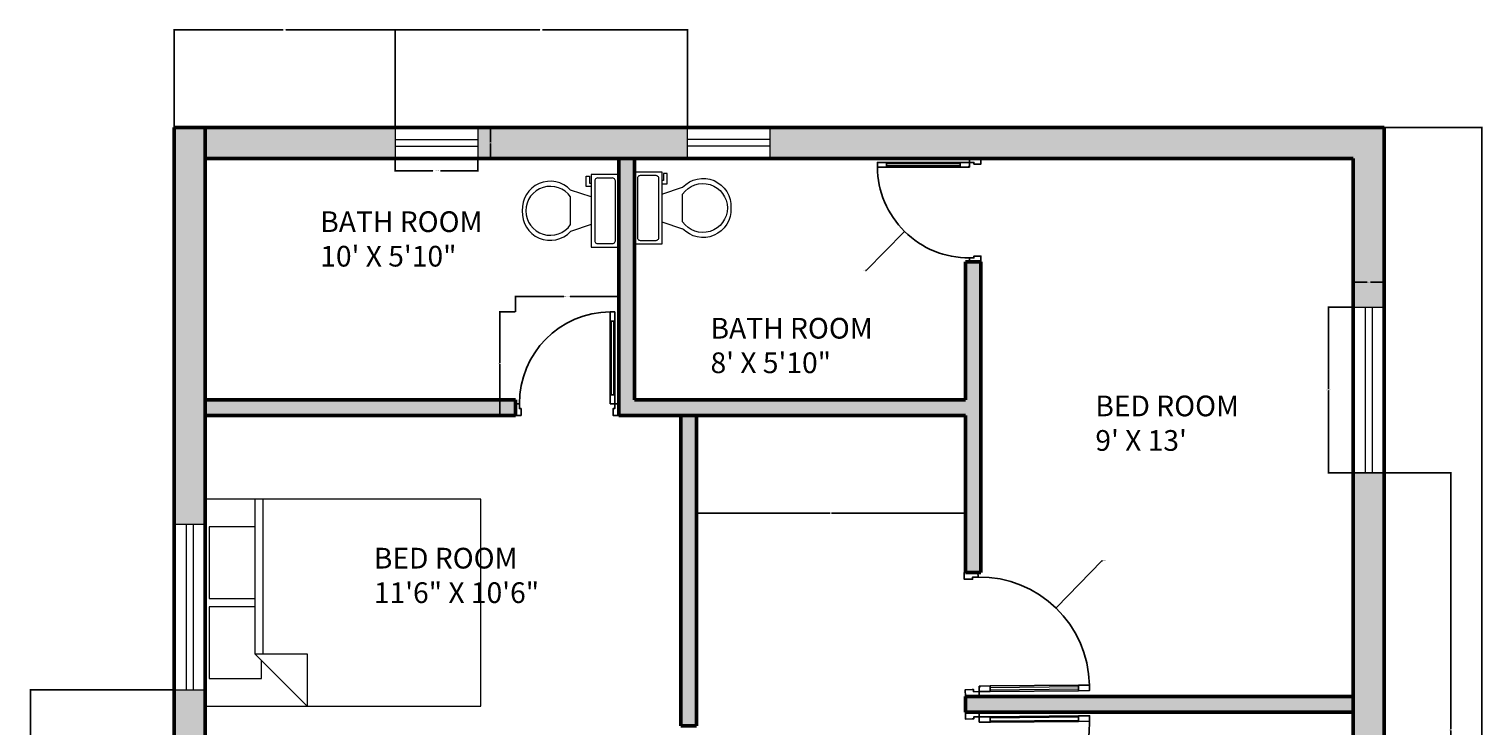
# Model space of a CAD drawing. Units: inches. Extents: x 5704 to 6126, y 2544 to 3123.
# Tile 2 of 2: x 5704 to 6126, y 2921 to 3123. Entities that reach past the tile are written whole.
import ezdxf

# ---------------------------------------------------------------- set-up
doc = ezdxf.new("R2010")
doc.units = ezdxf.units.IN
for name, color, linetype, lineweight in [('A-ANNO-DIMS', 2, 'Continuous', 18), ('A-AREA-IDEN', 7, 'Continuous', 18), ('A-Door', 150, 'Continuous', 25), ('A-FLOR-FIXT', 9, 'Continuous', 18), ('A-FURN', 8, 'Continuous', 18), ('A-Glaz', 92, 'Continuous', 18), ('A-WALL', 7, 'Continuous', 50)]:
    doc.layers.add(name, color=color, linetype=linetype, lineweight=lineweight)
doc.layers.add('A-WALL-PATT', color=18, linetype='Continuous', lineweight=13, true_color=0x000000)
doc.styles.get("Standard").update_dxf_attribs({"font": 'arial.ttf'})
doc.dimstyles.get("Standard").update_dxf_attribs({"dimtxt": 0.18, "dimasz": 0.18, "dimexe": 0.18, "dimexo": 0.0625, "dimgap": 0.09, "dimtad": 0, "dimtih": 1, "dimtoh": 1, "dimdec": 4, "dimzin": 0, "dimdsep": 46, "dimtxsty": 'Standard', "dimcen": 0.09, "dimadec": 0, "dimazin": 0, "dimtfac": 1, "dimtdec": 4, "dimtofl": 0, "dimtmove": 0, "dimatfit": 3, "dimfxl": 1, "dimtolj": 1, "dimtzin": 0, "dimarcsym": 0})

# ---------------------------------------------------------------- blocks, each defined once
blk = doc.blocks.new('A$C61230BBC')
blk.add_lwpolyline([(825, 180), (825, 820), (865, 820), (865, 180)], close=True)
blk.add_arc((830, 105), 795, 90.3603, 180.3603)
at = {"layer": 'A-Door'}
for points in [[(825, 900), (825, 820), (865, 820), (865, 900)], [(825, 100), (825, 180), (865, 180), (865, 100)], [(35, 100), (35, 60), (50, 60), (50, 50), (50, 0), (0, 0), (0, 100)], [(865, 100), (900, 100), (900, 0), (850, 0), (850, 50), (850, 60), (865, 60)]]:
    blk.add_lwpolyline(points, close=True, dxfattribs=at)
at = {"layer": 'A-Glaz'}
blk.add_lwpolyline([(835, 180), (835, 820), (855, 820), (855, 180)], close=True, dxfattribs=at)
blk = doc.blocks.new('*U3')
for p, q in [((9.5, -6), (9.5, -2)), ((-8, -8.5), (-8, -8)), ((-7, -8), (-7, -9.5)), ((-4, -8), (-6, -14)), ((4, -8), (6, -14)), ((-10, -8.5), (-8, -8.5)), ((-10, -9.5), (-10, -8.5)), ((-7, -9.5), (-10, -9.5)), ((4, -14), (-4, -14))]:
    blk.add_line(p, q)
blk.add_lwpolyline([(10.5, -8), (10.5, 0), (-10.5, 0), (-10.5, -8)], close=True)
for points in [[(-9.5, -2), (-9.5, -6)], [(8.5, -1), (-8.5, -1)], [(-8.5, -7), (8.5, -7)]]:
    blk.add_lwpolyline(points)
for centre, radius, start, end in [((-8.625, -1.875), 0.8839, 81.8699, 188.1301), ((8.625, -1.875), 0.8839, 351.8699, 98.1301), ((-8.625, -6.125), 0.8839, 171.869898, 278.1301), ((8.625, -6.125), 0.8839, 261.8699, 8.1301), ((-0.4772, -19.9188), 8.0953, 133.01722, 273.38), ((0.0374, -19.8731), 7.127, 124.50543, 269.7), ((-0.0373, -19.8731), 7.127, 270.3, 55.4946), ((0.4773, -19.9188), 8.0953, 266.62, 46.9828)]:
    blk.add_arc(centre, radius, start, end)
blk = doc.blocks.new('Bed - Queen')
for p, q in [((0, -80.00003), (0, 0)), ((0, 0), (59.99999, 0)), ((59.99999, 0), (59.99999, -80.00003)), ((7.99999, -1.2), (28.79998, -1.2)), ((7.99999, -14.4), (7.99999, -1.2)), ((28.79998, -1.2), (28.79998, -14.4)), ((31.19999, -1.2), (51.99999, -1.2)), ((31.19999, -14.4), (31.19999, -1.2)), ((51.99999, -1.2), (51.99999, -16.4)), ((0, -14.4), (44.8, -14.4)), ((44.8, -16.8), (0, -16.8)), ((59.99999, -29.6), (44.8, -14.4)), ((44.8, -14.4), (44.8, -29.6)), ((51.99999, -16.4), (46.79936, -16.4)), ((44.8, -29.6), (59.99999, -29.6)), ((59.99999, -80.00003), (0, -80.00003))]:
    blk.add_line(p, q)
blk = doc.blocks.new('WIN-24IN')
for p, q in [((0, 9), (0, 0)), ((24, 9), (24, 0)), ((0, 5.5), (24, 5.5)), ((0, 3.5), (24, 3.5))]:
    blk.add_line(p, q)
blk = doc.blocks.new('WIN-48IN')
for p, q in [((0, 48), (9, 48)), ((3.5, 48), (3.5, 0)), ((5.5, 48), (5.5, 0)), ((5.5, 48), (5.5, 0)), ((0, 0), (9, 0))]:
    blk.add_line(p, q)
blk = doc.blocks.new('*D8')
at = {"layer": 'A-ANNO-DIMS', "color": 0, "lineweight": -2, "transparency": 16777216}
for p, q in [((5845.44, 3040.68), (5845.44, 3045.3)), ((5845.62, 3045.12), (5859.5, 3045.12)), ((5875.26, 3045.12), (5861.37, 3045.12)), ((5875.44, 3040.68), (5875.44, 3045.3))]:
    blk.add_line(p, q, dxfattribs=at)
at = {"layer": 'A-ANNO-DIMS', "color": 0, "transparency": 16777216}
for points in [[(5845.62, 3045.15), (5845.62, 3045.09), (5845.44, 3045.12)], [(5875.26, 3045.15), (5875.26, 3045.09), (5875.44, 3045.12)]]:
    blk.add_solid(points, dxfattribs=at)
at = {"layer": 'Defpoints', "color": 0, "transparency": 16777216}
for p in [(5875.44, 3045.12), (5845.44, 3040.62), (5875.44, 3040.62)]:
    blk.add_point(p, dxfattribs=at)
at = {"layer": 'A-ANNO-DIMS', "color": 0, "transparency": 16777216, "insert": (5860.44, 3045.12), "char_height": 0.18, "attachment_point": 5}
blk.add_mtext('\\A1;DOOR 30 TYP.', dxfattribs=at)
blk = doc.blocks.new('*D9')
at = {"layer": 'A-ANNO-DIMS', "color": 0, "lineweight": -2, "transparency": 16777216}
for p, q in [((5845.37, 3040.62), (5840.76, 3040.62)), ((5840.94, 3040.44), (5840.94, 3025.8)), ((5840.94, 3010.8), (5840.94, 3025.44)), ((5845.37, 3010.62), (5840.76, 3010.62))]:
    blk.add_line(p, q, dxfattribs=at)
at = {"layer": 'A-ANNO-DIMS', "color": 0, "transparency": 16777216}
for points in [[(5840.91, 3040.44), (5840.97, 3040.44), (5840.94, 3040.62)], [(5840.91, 3010.8), (5840.97, 3010.8), (5840.94, 3010.62)]]:
    blk.add_solid(points, dxfattribs=at)
at = {"layer": 'Defpoints', "color": 0, "transparency": 16777216}
for p in [(5840.94, 3040.62), (5845.44, 3040.62), (5845.44, 3010.62)]:
    blk.add_point(p, dxfattribs=at)
at = {"layer": 'A-ANNO-DIMS', "color": 0, "transparency": 16777216, "insert": (5840.94, 3025.62), "char_height": 0.18, "attachment_point": 5}
blk.add_mtext('\\A1;30 TYP.', dxfattribs=at)
blk = doc.blocks.new('*D12')
at = {"layer": 'A-ANNO-DIMS', "color": 0, "lineweight": -2, "transparency": 16777216}
for p, q in [((5810.57, 3085.06), (5810.57, 3081.34)), ((5834.57, 3085.06), (5834.57, 3081.34)), ((5810.75, 3081.52), (5821.45, 3081.52)), ((5834.39, 3081.52), (5823.69, 3081.52))]:
    blk.add_line(p, q, dxfattribs=at)
at = {"layer": 'A-ANNO-DIMS', "color": 0, "transparency": 16777216}
for points in [[(5810.75, 3081.55), (5810.75, 3081.49), (5810.57, 3081.52)], [(5834.39, 3081.55), (5834.39, 3081.49), (5834.57, 3081.52)]]:
    blk.add_solid(points, dxfattribs=at)
at = {"layer": 'Defpoints', "color": 0, "transparency": 16777216}
for p in [(5810.57, 3085.12), (5834.57, 3085.12), (5834.57, 3081.52)]:
    blk.add_point(p, dxfattribs=at)
at = {"layer": 'A-ANNO-DIMS', "color": 0, "transparency": 16777216, "insert": (5822.57, 3081.52), "char_height": 0.18, "attachment_point": 5}
blk.add_mtext('\\A1;WINDOW 24 TYP.', dxfattribs=at)
blk = doc.blocks.new('*D13')
at = {"layer": 'A-ANNO-DIMS', "color": 0, "lineweight": -2, "transparency": 16777216}
for p, q in [((5834.63, 3094.12), (5838.35, 3094.12)), ((5838.17, 3093.94), (5838.17, 3089.8)), ((5838.17, 3085.3), (5838.17, 3089.44)), ((5834.63, 3085.12), (5838.35, 3085.12))]:
    blk.add_line(p, q, dxfattribs=at)
at = {"layer": 'A-ANNO-DIMS', "color": 0, "transparency": 16777216}
for points in [[(5838.14, 3093.94), (5838.2, 3093.94), (5838.17, 3094.12)], [(5838.14, 3085.3), (5838.2, 3085.3), (5838.17, 3085.12)]]:
    blk.add_solid(points, dxfattribs=at)
at = {"layer": 'Defpoints', "color": 0, "transparency": 16777216}
for p in [(5834.57, 3094.12), (5838.17, 3094.12), (5834.57, 3085.12)]:
    blk.add_point(p, dxfattribs=at)
at = {"layer": 'A-ANNO-DIMS', "color": 0, "transparency": 16777216, "insert": (5838.17, 3089.62), "char_height": 0.18, "attachment_point": 5}
blk.add_mtext('\\A1;9 TYP.', dxfattribs=at)
blk = doc.blocks.new('*D14')
at = {"layer": 'A-ANNO-DIMS', "color": 0, "lineweight": -2, "transparency": 16777216}
for p, q in [((6088.37, 3042.02), (6081.06, 3042.02)), ((6081.24, 3041.84), (6081.24, 3018.2)), ((6081.24, 2994.2), (6081.24, 3017.84)), ((6088.37, 2994.02), (6081.06, 2994.02))]:
    blk.add_line(p, q, dxfattribs=at)
at = {"layer": 'A-ANNO-DIMS', "color": 0, "transparency": 16777216}
for points in [[(6081.21, 3041.84), (6081.27, 3041.84), (6081.24, 3042.02)], [(6081.21, 2994.2), (6081.27, 2994.2), (6081.24, 2994.02)]]:
    blk.add_solid(points, dxfattribs=at)
at = {"layer": 'Defpoints', "color": 0, "transparency": 16777216}
for p in [(6081.24, 3042.02), (6088.44, 3042.02), (6088.44, 2994.02)]:
    blk.add_point(p, dxfattribs=at)
at = {"layer": 'A-ANNO-DIMS', "color": 0, "transparency": 16777216, "insert": (6081.24, 3018.02), "char_height": 0.18, "attachment_point": 5}
blk.add_mtext('\\A1;WINDOW 48 TYP.', dxfattribs=at)
blk = doc.blocks.new('*D15')
at = {"layer": 'A-ANNO-DIMS', "color": 0, "lineweight": -2, "transparency": 16777216}
for p, q in [((6088.44, 3042.08), (6088.44, 3049.4)), ((6088.62, 3049.22), (6092.48, 3049.22)), ((6097.26, 3049.22), (6093.39, 3049.22)), ((6097.44, 3042.08), (6097.44, 3049.4))]:
    blk.add_line(p, q, dxfattribs=at)
at = {"layer": 'A-ANNO-DIMS', "color": 0, "transparency": 16777216}
for points in [[(6088.62, 3049.25), (6088.62, 3049.19), (6088.44, 3049.22)], [(6097.26, 3049.25), (6097.26, 3049.19), (6097.44, 3049.22)]]:
    blk.add_solid(points, dxfattribs=at)
at = {"layer": 'Defpoints', "color": 0, "transparency": 16777216}
for p in [(6097.44, 3049.22), (6088.44, 3042.02), (6097.44, 3042.02)]:
    blk.add_point(p, dxfattribs=at)
at = {"layer": 'A-ANNO-DIMS', "color": 0, "transparency": 16777216, "insert": (6092.94, 3049.22), "char_height": 0.18, "attachment_point": 5}
blk.add_mtext('\\A1;9 TYP.', dxfattribs=at)
blk = doc.blocks.new('*D21')
at = {"layer": 'A-ANNO-DIMS', "color": 0, "lineweight": -2, "transparency": 16777216}
for p, q in [((6097.5, 3094.12), (6125.92, 3094.12)), ((6125.74, 3093.94), (6125.74, 2852.05)), ((6125.74, 2609.8), (6125.74, 2851.69)), ((6097.5, 2609.62), (6125.92, 2609.62))]:
    blk.add_line(p, q, dxfattribs=at)
at = {"layer": 'A-ANNO-DIMS', "color": 0, "transparency": 16777216}
for points in [[(6125.71, 3093.94), (6125.77, 3093.94), (6125.74, 3094.12)], [(6125.71, 2609.8), (6125.77, 2609.8), (6125.74, 2609.62)]]:
    blk.add_solid(points, dxfattribs=at)
at = {"layer": 'Defpoints', "color": 0, "transparency": 16777216}
for p in [(6097.44, 3094.12), (6125.74, 3094.12), (6097.44, 2609.62)]:
    blk.add_point(p, dxfattribs=at)
at = {"layer": 'A-ANNO-DIMS', "color": 0, "transparency": 16777216, "insert": (6125.74, 2851.87), "char_height": 0.18, "attachment_point": 5}
blk.add_mtext('\\A1;484.5', dxfattribs=at)
blk = doc.blocks.new('*D22')
at = {"layer": 'A-ANNO-DIMS', "color": 0, "lineweight": -2, "transparency": 16777216}
for p, q in [((5746.44, 3094.18), (5746.44, 3122.6)), ((5746.62, 3122.42), (5778.11, 3122.42)), ((5810.39, 3122.42), (5778.9, 3122.42)), ((5810.57, 3094.18), (5810.57, 3122.6))]:
    blk.add_line(p, q, dxfattribs=at)
at = {"layer": 'A-ANNO-DIMS', "color": 0, "transparency": 16777216}
for points in [[(5746.62, 3122.45), (5746.62, 3122.39), (5746.44, 3122.42)], [(5810.39, 3122.45), (5810.39, 3122.39), (5810.57, 3122.42)]]:
    blk.add_solid(points, dxfattribs=at)
at = {"layer": 'Defpoints', "color": 0, "transparency": 16777216}
for p in [(5810.57, 3122.42), (5746.44, 3094.12), (5810.57, 3094.12)]:
    blk.add_point(p, dxfattribs=at)
at = {"layer": 'A-ANNO-DIMS', "color": 0, "transparency": 16777216, "insert": (5778.5, 3122.42), "char_height": 0.18, "attachment_point": 5}
blk.add_mtext('\\A1;64.13', dxfattribs=at)
blk = doc.blocks.new('*D23')
at = {"layer": 'A-ANNO-DIMS', "color": 0, "lineweight": -2, "transparency": 16777216}
for p, q in [((5810.57, 3094.18), (5810.57, 3122.6)), ((5810.75, 3122.42), (5852.55, 3122.42)), ((5895.13, 3122.42), (5853.34, 3122.42)), ((5895.31, 3094.18), (5895.31, 3122.6))]:
    blk.add_line(p, q, dxfattribs=at)
at = {"layer": 'A-ANNO-DIMS', "color": 0, "transparency": 16777216}
for points in [[(5810.75, 3122.45), (5810.75, 3122.39), (5810.57, 3122.42)], [(5895.13, 3122.45), (5895.13, 3122.39), (5895.31, 3122.42)]]:
    blk.add_solid(points, dxfattribs=at)
at = {"layer": 'Defpoints', "color": 0, "transparency": 16777216}
for p in [(5895.31, 3122.42), (5810.57, 3094.12), (5895.31, 3094.12)]:
    blk.add_point(p, dxfattribs=at)
at = {"layer": 'A-ANNO-DIMS', "color": 0, "transparency": 16777216, "insert": (5852.94, 3122.42), "char_height": 0.18, "attachment_point": 5}
blk.add_mtext('\\A1;84.75', dxfattribs=at)
blk = doc.blocks.new('*D26')
at = {"layer": 'A-ANNO-DIMS', "color": 0, "lineweight": -2, "transparency": 16777216}
for p, q in [((5746.37, 2931.06), (5704.59, 2931.06)), ((5704.77, 2930.88), (5704.77, 2875.61)), ((5704.77, 2819.98), (5704.77, 2875.25)), ((5746.37, 2819.8), (5704.59, 2819.8))]:
    blk.add_line(p, q, dxfattribs=at)
at = {"layer": 'A-ANNO-DIMS', "color": 0, "transparency": 16777216}
for points in [[(5704.74, 2930.88), (5704.8, 2930.88), (5704.77, 2931.06)], [(5704.74, 2819.98), (5704.8, 2819.98), (5704.77, 2819.8)]]:
    blk.add_solid(points, dxfattribs=at)
at = {"layer": 'Defpoints', "color": 0, "transparency": 16777216}
for p in [(5704.77, 2931.06), (5746.44, 2931.06), (5746.44, 2819.8)]:
    blk.add_point(p, dxfattribs=at)
at = {"layer": 'A-ANNO-DIMS', "color": 0, "transparency": 16777216, "insert": (5704.77, 2875.43), "char_height": 0.18, "attachment_point": 5}
blk.add_mtext('\\A1;111.27', dxfattribs=at)
blk = doc.blocks.new('*D29')
at = {"layer": 'A-ANNO-DIMS', "color": 0, "lineweight": -2, "transparency": 16777216}
for p, q in [((6088.5, 2994.02), (6116.92, 2994.02)), ((6116.74, 2993.84), (6116.74, 2919.63)), ((6116.74, 2845.05), (6116.74, 2919.26)), ((6088.5, 2844.87), (6116.92, 2844.87))]:
    blk.add_line(p, q, dxfattribs=at)
at = {"layer": 'A-ANNO-DIMS', "color": 0, "transparency": 16777216}
for points in [[(6116.71, 2993.84), (6116.77, 2993.84), (6116.74, 2994.02)], [(6116.71, 2845.05), (6116.77, 2845.05), (6116.74, 2844.87)]]:
    blk.add_solid(points, dxfattribs=at)
at = {"layer": 'Defpoints', "color": 0, "transparency": 16777216}
for p in [(6088.44, 2994.02), (6088.44, 2844.87), (6116.74, 2844.87)]:
    blk.add_point(p, dxfattribs=at)
at = {"layer": 'A-ANNO-DIMS', "color": 0, "transparency": 16777216, "insert": (6116.74, 2919.45), "char_height": 0.18, "attachment_point": 5}
blk.add_mtext('\\A1;149.15', dxfattribs=at)
blk = doc.blocks.new('*D31')
at = {"layer": 'A-ANNO-DIMS', "color": 0, "lineweight": -2, "transparency": 16777216}
for p, q in [((5897.94, 3010.56), (5897.94, 2982.14)), ((5975.94, 3010.56), (5975.94, 2982.14)), ((5898.12, 2982.32), (5936.72, 2982.32)), ((5975.76, 2982.32), (5937.16, 2982.32))]:
    blk.add_line(p, q, dxfattribs=at)
at = {"layer": 'A-ANNO-DIMS', "color": 0, "transparency": 16777216}
for points in [[(5898.12, 2982.35), (5898.12, 2982.29), (5897.94, 2982.32)], [(5975.76, 2982.35), (5975.76, 2982.29), (5975.94, 2982.32)]]:
    blk.add_solid(points, dxfattribs=at)
at = {"layer": 'Defpoints', "color": 0, "transparency": 16777216}
for p in [(5897.94, 3010.62), (5975.94, 3010.62), (5897.94, 2982.32)]:
    blk.add_point(p, dxfattribs=at)
at = {"layer": 'A-ANNO-DIMS', "color": 0, "transparency": 16777216, "insert": (5936.94, 2982.32), "char_height": 0.18, "attachment_point": 5}
blk.add_mtext('\\A1;78', dxfattribs=at)
blk = doc.blocks.new('*D41')
at = {"layer": 'A-ANNO-DIMS', "color": 0, "lineweight": -2, "transparency": 16777216}
for p, q in [((6015.52, 2968.49), (6002.37, 2954.92)), ((6015.7, 2968.49), (6015.52, 2968.49)), ((5980.02, 2931.96), (5980.2, 2931.96)), ((5980.11, 2931.87), (5980.11, 2932.05))]:
    blk.add_line(p, q, dxfattribs=at)
at = {"layer": 'A-ANNO-DIMS', "color": 0, "transparency": 16777216}
blk.add_solid([(6002.35, 2954.94), (6002.39, 2954.9), (6002.24, 2954.79)], dxfattribs=at)
at = {"layer": 'Defpoints', "color": 0, "transparency": 16777216}
for p in [(6002.24, 2954.79), (5980.11, 2931.96)]:
    blk.add_point(p, dxfattribs=at)
at = {"layer": 'A-ANNO-DIMS', "color": 0, "transparency": 16777216, "insert": (6016.31, 2968.49), "char_height": 0.18, "attachment_point": 5}
blk.add_mtext('\\A1;4X R31.8', dxfattribs=at)
blk = doc.blocks.new('*D42')
at = {"layer": 'A-ANNO-DIMS', "color": 0, "lineweight": -2, "transparency": 16777216}
for p, q in [((5976.85, 3082.78), (5977.03, 3082.78)), ((5976.94, 3082.69), (5976.94, 3082.87)), ((5947.14, 3052.62), (5958.19, 3063.8)), ((5946.96, 3052.62), (5947.14, 3052.62))]:
    blk.add_line(p, q, dxfattribs=at)
at = {"layer": 'A-ANNO-DIMS', "color": 0, "transparency": 16777216}
blk.add_solid([(5958.17, 3063.82), (5958.21, 3063.78), (5958.32, 3063.93)], dxfattribs=at)
at = {"layer": 'Defpoints', "color": 0, "transparency": 16777216}
for p in [(5976.94, 3082.78), (5958.32, 3063.93)]:
    blk.add_point(p, dxfattribs=at)
at = {"layer": 'A-ANNO-DIMS', "color": 0, "transparency": 16777216, "insert": (5946.36, 3052.62), "char_height": 0.18, "attachment_point": 5}
blk.add_mtext('\\A1;3X R26.5', dxfattribs=at)

msp = doc.modelspace()

# ---------------------------------------------------------------- hatches: boundary and pattern name
at = {"layer": 'A-WALL-PATT'}
h = msp.add_hatch(color=256, dxfattribs=at)
h.dxf.hatch_style = 1
h.paths.add_polyline_path([(5755.4367, 2734.6788), (5746.4367, 2734.6788), (5746.4367, 2694.1938), (5755.4367, 2694.1938)])
h.paths.add_polyline_path([(5755.4367, 2931.063), (5746.4367, 2931.063), (5746.4367, 2843.7971), (5755.4367, 2843.7971)])
h.paths.add_polyline_path([(5755.4367, 3094.1182), (5746.4367, 3094.1182), (5746.4367, 2979.063), (5755.4367, 2979.063)])
h.paths.add_polyline_path([(5810.5679, 3094.1182), (5755.4367, 3094.1182), (5755.4367, 3085.1182), (5810.5679, 3085.1182)])
h.paths.add_polyline_path([(5895.3146, 3094.1182), (5834.5679, 3094.1182), (5834.5679, 3085.1182), (5895.3146, 3085.1182)])
h.paths.add_polyline_path([(6097.4367, 3094.1182), (5919.3146, 3094.1182), (5919.3146, 3085.1182), (6088.4367, 3085.1182), (6088.4367, 3042.019), (6097.4367, 3042.019), (6097.4367, 3085.1182)])
h.paths.add_polyline_path([(6097.4367, 2994.019), (6088.4367, 2994.019), (6088.4367, 2892.8723), (6097.4367, 2892.8723)])
h.paths.add_polyline_path([(6097.4367, 2844.8723), (6088.4367, 2844.8723), (6088.4367, 2740.0934), (6097.4367, 2740.0934)])
h = msp.add_hatch(color=256, dxfattribs=at)
h.dxf.hatch_style = 1
h.paths.add_polyline_path([(5980.4367, 3055.1182), (5975.9367, 3055.1182), (5975.9367, 3015.1182), (5879.9367, 3015.1182), (5879.9367, 3085.1182), (5875.4367, 3085.1182), (5875.4367, 3010.6182), (5879.9367, 3010.6182), (5975.9367, 3010.6182), (5975.9367, 2965.1182), (5980.4367, 2965.1182)])
h.paths.add_polyline_path([(5897.9367, 3010.6182), (5893.4367, 3010.6182), (5893.4367, 2920.6182), (5897.9367, 2920.6182)])
h.paths.add_polyline_path([(5845.4367, 3015.1182), (5755.4367, 3015.1182), (5755.4367, 3010.6182), (5845.4367, 3010.6182)])
h.paths.add_polyline_path([(5897.9367, 2884.6182), (5845.4367, 2884.6182), (5755.4367, 2884.6182), (5755.4367, 2880.1182), (5845.4367, 2880.1182), (5897.9367, 2880.1182)])
h.paths.add_polyline_path([(5843.9367, 2880.1182), (5839.4367, 2880.1182), (5839.4367, 2822.3967), (5843.9367, 2822.3967)])
h.paths.add_polyline_path([(5922.4367, 2707.6182), (5897.9367, 2707.6182), (5845.4367, 2707.6182), (5755.4367, 2707.6182), (5755.4367, 2698.6182), (5845.4367, 2698.6182), (5897.9367, 2698.6182), (5922.4367, 2698.6182)])
h.paths.add_polyline_path([(5897.9367, 2784.1182), (5845.4367, 2784.1182), (5755.4367, 2784.1182), (5755.4367, 2779.6182), (5845.4367, 2779.6182), (5897.9367, 2779.6182)])
h = msp.add_hatch(color=256, dxfattribs=at)
h.dxf.hatch_style = 1
h.paths.add_polyline_path([(5988.7946, 2707.6182), (5958.4367, 2707.6182), (5958.5117, 2703.6189), (5958.4367, 2703.6175), (5958.4367, 2618.6182), (5958.4367, 2609.6182), (6097.4367, 2609.6182), (6097.4367, 2716.0934), (6088.4367, 2716.0934), (6088.4367, 2618.6182), (5962.9367, 2618.6182), (5962.9367, 2698.6182), (5988.7946, 2698.6182)])
h.paths.add_polyline_path([(5980.4367, 2888.6182), (5975.9367, 2888.6182), (5975.9367, 2764.1182), (5980.4367, 2764.1182), (6088.4367, 2764.1182), (6088.4367, 2768.6182), (5980.4367, 2768.6182)])
h.paths.add_polyline_path([(6088.4367, 2929.1182), (5980.4367, 2929.1182), (5975.9367, 2929.1182), (5975.9367, 2924.6182), (5980.4367, 2924.6182), (6088.4367, 2924.6182)])

# ---------------------------------------------------------------- linework, layer by layer
at = {"layer": 'A-WALL'}
for p, q in [((5746.4367, 3094.1182), (6097.4367, 3094.1182)), ((5746.4367, 3094.1182), (5746.4367, 2609.6182)), ((5755.4367, 3094.1182), (5755.4367, 2694.1938)), ((6097.4367, 3085.1182), (6097.4367, 3094.1182)), ((5755.4367, 3085.1182), (6088.4367, 3085.1182)), ((5875.4367, 3085.1182), (5875.4367, 3010.6182)), ((5879.9367, 3085.1182), (5879.9367, 3015.1182)), ((6088.4367, 3085.1182), (6088.4367, 2618.6182)), ((6097.4367, 3085.1182), (6097.4367, 2609.6182)), ((5975.9367, 3055.1182), (5975.9367, 3015.1182)), ((5975.9367, 3055.1182), (5980.4367, 3055.1182)), ((5980.4367, 3055.1182), (5980.4367, 2965.1182)), ((5755.4367, 3015.1182), (5845.4367, 3015.1182)), ((5845.4367, 3015.1182), (5845.4367, 3010.6182)), ((5879.9367, 3015.1182), (5975.9367, 3015.1182)), ((5755.4367, 3010.6182), (5845.4367, 3010.6182)), ((5879.9367, 3010.6182), (5875.4367, 3010.6182)), ((5879.9367, 3010.6182), (5975.9367, 3010.6182)), ((5893.4367, 3010.6182), (5893.4367, 2920.6182)), ((5897.9367, 3010.6182), (5897.9367, 2920.6182)), ((5975.9367, 3010.6182), (5975.9367, 2965.1182)), ((5980.4367, 2965.1182), (5975.9367, 2965.1182)), ((5980.4367, 2929.1182), (5975.9367, 2929.1182)), ((5975.9367, 2929.1182), (5975.9367, 2924.6182)), ((5975.9367, 2929.1182), (5975.9367, 2924.6182)), ((5980.4367, 2929.1182), (6088.4367, 2929.1182)), ((5980.4367, 2924.6182), (5975.9367, 2924.6182)), ((5980.4367, 2924.6182), (6088.4367, 2924.6182)), ((5893.4367, 2920.6182), (5897.9367, 2920.6182))]:
    msp.add_line(p, q, dxfattribs=at)

# ---------------------------------------------------------------- block references
at = {"layer": 'A-Door'}
for p, xscale, yscale, zscale, rotation in [((5980.4367, 3055.1182), 0.0333333333333333, 0.0333333333333333, 0.0333333333333333, 90), ((5975.5993, 2965.1167), 0.0399999999200469, 0.0399999999200469, 0.0399999999200469, 270.5370384371627), ((5976.2741, 2888.6198), -0.0399999999200469, 0.0399999999200469, 0.0399999999200469, 270.5370384371518)]:
    msp.add_blockref('A$C61230BBC', p, dxfattribs=dict(at, xscale=xscale, yscale=yscale, zscale=zscale, rotation=rotation))
at = {"layer": 'A-Door', "xscale": 0.0333333333333333, "yscale": 0.0333333333333333, "zscale": 0.0333333333333333}
msp.add_blockref('A$C61230BBC', (5845.4367, 3010.6182), dxfattribs=at)
at = {"layer": 'A-FLOR-FIXT', "rotation": 270}
msp.add_blockref('*U3', (5875.4367, 3069.9305), dxfattribs=at)
at = {"layer": 'A-FLOR-FIXT', "xscale": -1, "rotation": 90}
msp.add_blockref('*U3', (5879.9367, 3070.745), dxfattribs=at)
at = {"layer": 'A-FURN', "xscale": -1, "rotation": 90}
msp.add_blockref('Bed - Queen', (5755.4367, 2986.3235), dxfattribs=at)
at = {"layer": 'A-Glaz'}
for name, p in [('WIN-24IN', (5810.568, 3085.118)), ('WIN-48IN', (6088.437, 2994.0189)), ('WIN-48IN', (5746.437, 2931.063))]:
    msp.add_blockref(name, p, dxfattribs=at)
at = {"layer": 'A-Glaz', "rotation": 180}
msp.add_blockref('WIN-24IN', (5919.3145, 3094.1185), dxfattribs=at)

# ---------------------------------------------------------------- texts
at = {"layer": 'A-AREA-IDEN', "char_height": 6, "attachment_point": 1}
for s, insert in [('BATH ROOM\\P10\' X 5\'10"', (5788.8443, 3069.7706)), ('BATH ROOM\\P8\' X 5\'10"', (5902.0283, 3038.8796)), ("BED ROOM\\P9' X 13'", (6013.6404, 3016.3634)), ('BED ROOM\\P11\'6" X 10\'6"', (5804.3935, 2972.2416))]:
    msp.add_mtext_dynamic_manual_height_columns(s, width=70.528111, gutter_width=12.5, heights=[0], dxfattribs=dict(at, insert=insert))

# ---------------------------------------------------------------- dimensions: what is measured, and where the dimension line sits
at = {"layer": 'A-ANNO-DIMS'}
for base, p1, p2, picture, middle in [((5810.5679, 3122.4182), (5746.4367, 3094.1182), (5810.5679, 3094.1182), '*D22', (5778.5023, 3122.4182)), ((5895.3146, 3122.4182), (5810.5679, 3094.1182), (5895.3146, 3094.1182), '*D23', (5852.9412, 3122.4182))]:
    dim = msp.add_linear_dim(base=base, p1=p1, p2=p2, dimstyle='Standard', override={"dimdec": 2, "dimlfac": 1, "dimrnd": 0, "dimzin": 0, "dimdsep": 46, "dimlunit": 2}, dxfattribs=at)
    dim.commit()
    dim.dimension.update_dxf_attribs({"geometry": picture, "text_midpoint": middle})
for base, p1, p2, text, picture, middle in [((5838.1679, 3094.1182), (5834.5679, 3085.1182), (5834.5679, 3094.1182), '<> TYP.', '*D13', (5838.1679, 3089.6182)), ((5840.9367, 3040.6182), (5845.4367, 3010.6182), (5845.4367, 3040.6182), '<> TYP.', '*D9', (5840.9367, 3025.6182)), ((6081.2367, 3042.019), (6088.4367, 2994.019), (6088.4367, 3042.019), 'WINDOW <> TYP.', '*D14', (6081.2367, 3018.019))]:
    dim = msp.add_linear_dim(base=base, p1=p1, p2=p2, angle=90, text=text, dimstyle='Standard', override={"dimdec": 0, "dimlfac": 1, "dimrnd": 0, "dimzin": 0, "dimdsep": 46, "dimlunit": 2}, dxfattribs=at)
    dim.commit()
    dim.dimension.update_dxf_attribs({"geometry": picture, "text_midpoint": middle})
for base, p1, p2, angle, override, picture, middle in [((6125.7367, 3094.1182), (6097.4367, 2609.6182), (6097.4367, 3094.1182), 90, {"dimdec": 1, "dimlfac": 1, "dimrnd": 0, "dimzin": 0, "dimdsep": 46, "dimlunit": 2}, '*D21', (6125.7367, 2851.8682)), ((5897.9367, 2982.3182), (5975.9367, 3010.6182), (5897.9367, 3010.6182), 180, {"dimdec": 0, "dimlfac": 1, "dimrnd": 0, "dimzin": 0, "dimdsep": 46, "dimlunit": 2}, '*D31', (5936.9367, 2982.3182)), ((6116.7367, 2844.8723), (6088.4367, 2994.019), (6088.4367, 2844.8723), 270, {"dimdec": 2, "dimlfac": 1, "dimrnd": 0, "dimzin": 0, "dimdsep": 46, "dimlunit": 2}, '*D29', (6116.7367, 2919.4456)), ((5704.7677, 2931.063), (5746.4367, 2819.7971), (5746.4367, 2931.063), 90, {"dimdec": 2, "dimlfac": 1, "dimrnd": 0, "dimzin": 0, "dimdsep": 46, "dimlunit": 2}, '*D26', (5704.7677, 2875.4301))]:
    dim = msp.add_linear_dim(base=base, p1=p1, p2=p2, angle=angle, dimstyle='Standard', override=override, dxfattribs=at)
    dim.commit()
    dim.dimension.update_dxf_attribs({"geometry": picture, "text_midpoint": middle})
for base, p1, p2, text, picture, middle in [((5834.5679, 3081.5182), (5810.5679, 3085.1182), (5834.5679, 3085.1182), 'WINDOW <> TYP.', '*D12', (5822.5679, 3081.5182)), ((6097.4367, 3049.219), (6088.4367, 3042.019), (6097.4367, 3042.019), '<> TYP.', '*D15', (6092.9367, 3049.219)), ((5875.4367, 3045.1182), (5845.4367, 3040.6182), (5875.4367, 3040.6182), 'DOOR <> TYP.', '*D8', (5860.4367, 3045.1182))]:
    dim = msp.add_linear_dim(base=base, p1=p1, p2=p2, text=text, dimstyle='Standard', override={"dimdec": 0, "dimlfac": 1, "dimrnd": 0, "dimzin": 0, "dimdsep": 46, "dimlunit": 2}, dxfattribs=at)
    dim.commit()
    dim.dimension.update_dxf_attribs({"geometry": picture, "text_midpoint": middle})
for center, mpoint, text, picture, middle in [((5976.9367, 3082.7849), (5958.316, 3063.929), '3X <>', '*D42', (5946.3596, 3052.6154)), ((5980.1103, 2931.9575), (6002.2421, 2954.7931), '4X <>', '*D41', (6016.3082, 2968.4944))]:
    dim = msp.add_radius_dim(center=center, mpoint=mpoint, text=text, dimstyle='Standard', override={"dimdec": 1, "dimlfac": 1, "dimrnd": 0, "dimzin": 0, "dimdsep": 46, "dimlunit": 2}, dxfattribs=at)
    dim.commit()
    dim.dimension.update_dxf_attribs({"geometry": picture, "text_midpoint": middle, "dimtype": 164})

doc.saveas('drawing.dxf')
